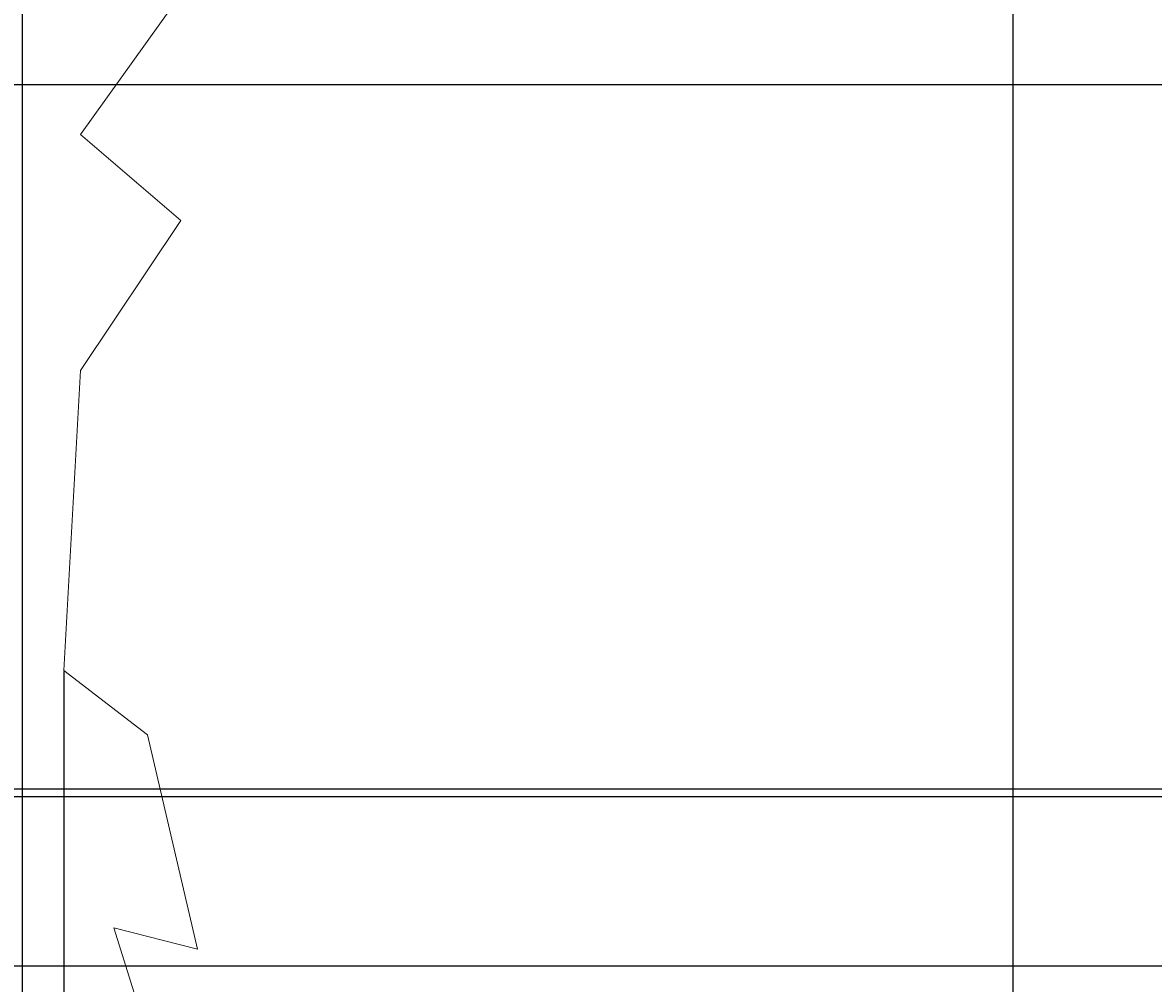
# Model space of a CAD drawing. Units: inches. Extents: x -26 to 776, y -22 to 650.
# Tile 47 of 62: x 426 to 506, y 158 to 226. Entities that reach past the tile are written whole.
import ezdxf

# ---------------------------------------------------------------- set-up
doc = ezdxf.new("R2010")
doc.units = ezdxf.units.IN
doc.header["$MEASUREMENT"] = 0
doc.layers.add('A-ANNO-DIMS', color=2, linetype='Continuous', lineweight=18)
doc.layers.add('L-PLNT-TREE', color=94, linetype='Continuous', lineweight=18)
doc.styles.get("Standard").update_dxf_attribs({"font": 'arial.ttf'})
doc.dimstyles.get("Standard").update_dxf_attribs({"dimtxt": 0.5625, "dimasz": 0.18, "dimexe": 0.18, "dimexo": 0.0625, "dimgap": 0.09, "dimtad": 0, "dimtih": 1, "dimtoh": 1, "dimdec": 4, "dimzin": 0, "dimdsep": 46, "dimlunit": 4, "dimtxsty": 'Standard', "dimcen": 0.09, "dimadec": 0, "dimazin": 0, "dimtfac": 1, "dimtdec": 4, "dimtofl": 0, "dimtmove": 0, "dimatfit": 3, "dimfxl": 1, "dimtolj": 1, "dimtzin": 0, "dimarcsym": 0})

# ---------------------------------------------------------------- blocks, each defined once
blk = doc.blocks.new('Tree - type 2 deciduous elevation')
blk.add_lwpolyline([(-34.386, 107.646), (-40.712, 98.798), (-37.261, 95.849), (-40.712, 90.688), (-41.287, 80.366), (-38.412, 78.154), (-36.686, 70.781), (-39.562, 71.518), (-37.261, 64.145), (-38.412, 57.509), (-36.111, 58.247), (-33.236, 52.348), (-35.536, 53.086), (-34.961, 46.45), (-30.36, 44.975), (-31.51, 36.128)])
blk = doc.blocks.new('*D20')
at = {"layer": 'A-ANNO-DIMS', "color": 0, "lineweight": -2, "transparency": 16777216}
for p, q in [((425.806, 455.472), (775.335, 455.472)), ((775.155, 455.292), (775.155, 235.854)), ((775.155, 15.662), (775.155, 235.1)), ((425.806, 15.482), (775.335, 15.482))]:
    blk.add_line(p, q, dxfattribs=at)
at = {"layer": 'A-ANNO-DIMS', "color": 0, "transparency": 16777216}
for points in [[(775.125, 455.292), (775.185, 455.292), (775.155, 455.472)], [(775.125, 15.662), (775.185, 15.662), (775.155, 15.482)]]:
    blk.add_solid(points, dxfattribs=at)
at = {"layer": 'Defpoints', "color": 0, "transparency": 16777216}
for p in [(425.743, 455.472), (775.155, 455.472), (425.743, 15.482)]:
    blk.add_point(p, dxfattribs=at)
at = {"layer": 'A-ANNO-DIMS', "color": 0, "transparency": 16777216, "insert": (775.155, 235.477), "char_height": 0.5625, "attachment_point": 5}
blk.add_mtext('\\A1;440', dxfattribs=at)
blk = doc.blocks.new('*D26')
at = {"layer": 'A-ANNO-DIMS', "color": 0, "lineweight": -2, "transparency": 16777216}
for p, q in [((91.707, 171.973), (775.335, 171.973)), ((775.155, 171.793), (775.155, 166.105)), ((775.155, 159.662), (775.155, 165.351)), ((82.196, 159.482), (775.335, 159.482))]:
    blk.add_line(p, q, dxfattribs=at)
at = {"layer": 'A-ANNO-DIMS', "color": 0, "transparency": 16777216}
for points in [[(775.125, 171.793), (775.185, 171.793), (775.155, 171.973)], [(775.125, 159.662), (775.185, 159.662), (775.155, 159.482)]]:
    blk.add_solid(points, dxfattribs=at)
at = {"layer": 'Defpoints', "color": 0, "transparency": 16777216}
for p in [(91.645, 171.973), (775.155, 171.973), (82.134, 159.482)]:
    blk.add_point(p, dxfattribs=at)
at = {"layer": 'A-ANNO-DIMS', "color": 0, "transparency": 16777216, "insert": (775.155, 165.728), "char_height": 0.5625, "attachment_point": 5}
blk.add_mtext('\\A1;12.49', dxfattribs=at)
blk = doc.blocks.new('*D28')
at = {"layer": 'A-ANNO-DIMS', "color": 0, "lineweight": -2, "transparency": 16777216}
for p, q in [((285.08, 314.119), (775.335, 314.119)), ((775.155, 313.939), (775.155, 243.141)), ((775.155, 171.597), (775.155, 242.396)), ((285.08, 171.417), (775.335, 171.417))]:
    blk.add_line(p, q, dxfattribs=at)
at = {"layer": 'A-ANNO-DIMS', "color": 0, "transparency": 16777216}
for points in [[(775.125, 313.939), (775.185, 313.939), (775.155, 314.119)], [(775.125, 171.597), (775.185, 171.597), (775.155, 171.417)]]:
    blk.add_solid(points, dxfattribs=at)
at = {"layer": 'Defpoints', "color": 0, "transparency": 16777216}
for p in [(285.018, 314.119), (775.155, 314.119), (285.018, 171.417)]:
    blk.add_point(p, dxfattribs=at)
at = {"layer": 'A-ANNO-DIMS', "color": 0, "transparency": 16777216, "insert": (775.155, 242.768), "char_height": 0.5625, "attachment_point": 5}
blk.add_mtext('\\A1;142.7', dxfattribs=at)
blk = doc.blocks.new('*D39')
at = {"layer": 'A-ANNO-DIMS', "color": 0, "lineweight": -2, "transparency": 16777216}
for p, q in [((289.242, 15.545), (289.242, 649.856)), ((289.422, 649.676), (356.478, 649.676)), ((425.563, 649.676), (358.508, 649.676)), ((425.743, 15.545), (425.743, 649.856))]:
    blk.add_line(p, q, dxfattribs=at)
at = {"layer": 'A-ANNO-DIMS', "color": 0, "transparency": 16777216}
for points in [[(289.422, 649.706), (289.422, 649.646), (289.242, 649.676)], [(425.563, 649.706), (425.563, 649.646), (425.743, 649.676)]]:
    blk.add_solid(points, dxfattribs=at)
at = {"layer": 'Defpoints', "color": 0, "transparency": 16777216}
for p in [(425.743, 649.676), (289.242, 15.482), (425.743, 15.482)]:
    blk.add_point(p, dxfattribs=at)
at = {"layer": 'A-ANNO-DIMS', "color": 0, "transparency": 16777216, "insert": (357.493, 649.676), "char_height": 0.5625, "attachment_point": 5}
blk.add_mtext('\\A1;136.5', dxfattribs=at)
blk = doc.blocks.new('*D40')
at = {"layer": 'A-ANNO-DIMS', "color": 0, "lineweight": -2, "transparency": 16777216}
for p, q in [((425.743, 15.545), (425.743, 649.856)), ((425.923, 649.676), (459.646, 649.676)), ((495.451, 649.676), (461.728, 649.676)), ((495.631, 15.545), (495.631, 649.856))]:
    blk.add_line(p, q, dxfattribs=at)
at = {"layer": 'A-ANNO-DIMS', "color": 0, "transparency": 16777216}
for points in [[(425.923, 649.706), (425.923, 649.646), (425.743, 649.676)], [(495.451, 649.706), (495.451, 649.646), (495.631, 649.676)]]:
    blk.add_solid(points, dxfattribs=at)
at = {"layer": 'Defpoints', "color": 0, "transparency": 16777216}
for p in [(495.631, 649.676), (425.743, 15.482), (495.631, 15.482)]:
    blk.add_point(p, dxfattribs=at)
at = {"layer": 'A-ANNO-DIMS', "color": 0, "transparency": 16777216, "insert": (460.687, 649.676), "char_height": 0.5625, "attachment_point": 5}
blk.add_mtext('\\A1;69.89', dxfattribs=at)
blk = doc.blocks.new('*D41')
at = {"layer": 'A-ANNO-DIMS', "color": 0, "lineweight": -2, "transparency": 16777216}
for p, q in [((11.17, 221.641), (775.335, 221.641)), ((775.155, 221.461), (775.155, 190.939)), ((775.155, 159.662), (775.155, 190.185)), ((11.17, 159.482), (775.335, 159.482))]:
    blk.add_line(p, q, dxfattribs=at)
at = {"layer": 'A-ANNO-DIMS', "color": 0, "transparency": 16777216}
for points in [[(775.125, 221.461), (775.185, 221.461), (775.155, 221.641)], [(775.125, 159.662), (775.185, 159.662), (775.155, 159.482)]]:
    blk.add_solid(points, dxfattribs=at)
at = {"layer": 'Defpoints', "color": 0, "transparency": 16777216}
for p in [(11.107, 221.641), (775.155, 221.641), (11.107, 159.482)]:
    blk.add_point(p, dxfattribs=at)
at = {"layer": 'A-ANNO-DIMS', "color": 0, "transparency": 16777216, "insert": (775.155, 190.562), "char_height": 0.5625, "attachment_point": 5}
blk.add_mtext('\\A1;62.16', dxfattribs=at)
blk = doc.blocks.new('*D42')
at = {"layer": 'A-ANNO-DIMS', "color": 0, "lineweight": -2, "transparency": 16777216}
for p, q in [((285.08, 171.417), (775.335, 171.417)), ((775.155, 171.237), (775.155, 165.827)), ((775.155, 159.662), (775.155, 165.072)), ((289.305, 159.482), (775.335, 159.482))]:
    blk.add_line(p, q, dxfattribs=at)
at = {"layer": 'A-ANNO-DIMS', "color": 0, "transparency": 16777216}
for points in [[(775.125, 171.237), (775.185, 171.237), (775.155, 171.417)], [(775.125, 159.662), (775.185, 159.662), (775.155, 159.482)]]:
    blk.add_solid(points, dxfattribs=at)
at = {"layer": 'Defpoints', "color": 0, "transparency": 16777216}
for p in [(285.018, 171.417), (775.155, 171.417), (289.242, 159.482)]:
    blk.add_point(p, dxfattribs=at)
at = {"layer": 'A-ANNO-DIMS', "color": 0, "transparency": 16777216, "insert": (775.155, 165.45), "char_height": 0.5625, "attachment_point": 5}
blk.add_mtext('\\A1;11.935', dxfattribs=at)
blk = doc.blocks.new('*D47')
at = {"layer": 'A-ANNO-DIMS', "color": 0, "lineweight": -2, "transparency": 16777216}
for p, q in [((584.343, 199.901), (584.343, -21.315)), ((428.648, 180.243), (428.648, -21.315)), ((428.828, -21.135), (505.483, -21.135)), ((584.163, -21.135), (507.508, -21.135))]:
    blk.add_line(p, q, dxfattribs=at)
at = {"layer": 'A-ANNO-DIMS', "color": 0, "transparency": 16777216}
for points in [[(428.828, -21.105), (428.828, -21.165), (428.648, -21.135)], [(584.163, -21.105), (584.163, -21.165), (584.343, -21.135)]]:
    blk.add_solid(points, dxfattribs=at)
at = {"layer": 'Defpoints', "color": 0, "transparency": 16777216}
for p in [(584.343, 199.963), (428.648, 180.305), (584.343, -21.135)]:
    blk.add_point(p, dxfattribs=at)
at = {"layer": 'A-ANNO-DIMS', "color": 0, "transparency": 16777216, "insert": (506.496, -21.135), "char_height": 0.5625, "attachment_point": 5}
blk.add_mtext('\\A1;155.7', dxfattribs=at)

msp = doc.modelspace()

# ---------------------------------------------------------------- block references
at = {"layer": 'L-PLNT-TREE', "xscale": 2.050905272406618, "yscale": 2.050905272406618, "zscale": 2.050905272406618}
msp.add_blockref('Tree - type 2 deciduous elevation', (513.3241, 15.4824), dxfattribs=at)

# ---------------------------------------------------------------- dimensions: what is measured, and where the dimension line sits
at = {"layer": 'A-ANNO-DIMS'}
for base, p1, p2, override, picture, middle in [((425.7434, 649.6763), (289.2424, 15.4824), (425.7434, 15.4824), {"dimdec": 1, "dimlfac": 1, "dimrnd": 0, "dimzin": 0, "dimdsep": 46, "dimlunit": 2}, '*D39', (357.4929, 649.6763)), ((495.6309, 649.6763), (425.7434, 15.4824), (495.6309, 15.4824), {"dimdec": 2, "dimlfac": 1, "dimrnd": 0, "dimzin": 0, "dimdsep": 46, "dimlunit": 2}, '*D40', (460.6872, 649.6763)), ((584.3428, -21.1349), (428.6484, 180.3054), (584.3428, 199.9634), {"dimdec": 1, "dimlfac": 1, "dimrnd": 0, "dimzin": 0, "dimdsep": 46, "dimlunit": 2}, '*D47', (506.4956, -21.1349))]:
    dim = msp.add_linear_dim(base=base, p1=p1, p2=p2, dimstyle='Standard', override=override, dxfattribs=at)
    dim.commit()
    dim.dimension.update_dxf_attribs({"geometry": picture, "text_midpoint": middle})
for base, p1, p2, override, picture, middle in [((775.1553, 455.4717), (425.7434, 15.4824), (425.7434, 455.4717), {"dimdec": 0, "dimlfac": 1, "dimrnd": 0, "dimzin": 0, "dimdsep": 46, "dimlunit": 2}, '*D20', (775.1553, 235.477)), ((775.1553, 314.119), (285.0179, 171.4173), (285.0179, 314.119), {"dimdec": 1, "dimlfac": 1, "dimrnd": 0, "dimzin": 0, "dimdsep": 46, "dimlunit": 2}, '*D28', (775.1553, 242.7682)), ((775.1553, 221.6413), (11.1074, 159.4824), (11.1074, 221.6413), {"dimdec": 2, "dimlfac": 1, "dimrnd": 0, "dimzin": 0, "dimdsep": 46, "dimlunit": 2}, '*D41', (775.1553, 190.5618)), ((775.1553, 171.9734), (82.134, 159.4824), (91.6448, 171.9734), {"dimdec": 2, "dimlfac": 1, "dimrnd": 0, "dimzin": 0, "dimdsep": 46, "dimlunit": 2}, '*D26', (775.1553, 165.7279)), ((775.1553, 171.4173), (289.2424, 159.4824), (285.0179, 171.4173), {"dimdec": 3, "dimlfac": 1, "dimrnd": 0, "dimzin": 0, "dimdsep": 46, "dimlunit": 2}, '*D42', (775.1553, 165.4498))]:
    dim = msp.add_linear_dim(base=base, p1=p1, p2=p2, angle=90, dimstyle='Standard', override=override, dxfattribs=at)
    dim.commit()
    dim.dimension.update_dxf_attribs({"geometry": picture, "text_midpoint": middle})

doc.saveas('drawing.dxf')
